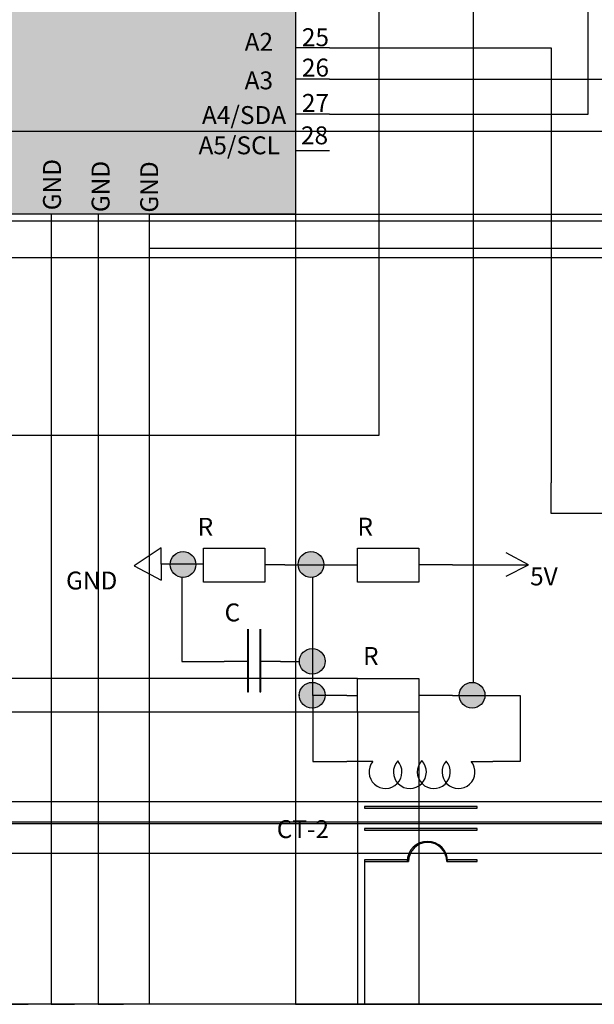
# Model space of a CAD drawing. Units: inches. Extents: x 35362 to 73946, y 43607 to 67532.
# Tile 133 of 134: x 57838 to 64925, y 43607 to 55752. Entities that reach past the tile are written whole.
import ezdxf

# ---------------------------------------------------------------- set-up
doc = ezdxf.new("R2010")
doc.units = ezdxf.units.IN
doc.header["$MEASUREMENT"] = 0
for name, color, linetype, lineweight in [('A-ANNO-DIMS', 2, 'Continuous', 18), ('E-ANNO-TEXT', 5, 'Continuous', 18), ('E-SYMB', 1, 'Continuous', 25), ('E-SYMB-PATT', 1, 'Continuous', 13), ('E-WIRE', 3, 'Continuous', 25)]:
    doc.layers.add(name, color=color, linetype=linetype, lineweight=lineweight)
doc.styles.get("Standard").update_dxf_attribs({"font": 'arial.ttf'})
doc.dimstyles.get("Standard").update_dxf_attribs({"dimtxt": 0.18, "dimasz": 0.18, "dimexe": 0.18, "dimexo": 0.0625, "dimgap": 0.09, "dimtad": 0, "dimtih": 1, "dimtoh": 1, "dimdec": 4, "dimzin": 0, "dimdsep": 46, "dimtxsty": 'Standard', "dimcen": 0.09, "dimadec": 0, "dimazin": 0, "dimtfac": 1, "dimtdec": 4, "dimtofl": 0, "dimtmove": 0, "dimatfit": 3, "dimfxl": 1, "dimtolj": 1, "dimtzin": 0, "dimarcsym": 0})

# ---------------------------------------------------------------- blocks, each defined once
blk = doc.blocks.new('CT-CORE')
for p, q in [((-0.0004610742907971, 1387.996120092102), (-0.0004610742907971, -5.34733626409e-05)), ((19.99953892572375, 1387.996120092102), (-0.0004610742907971, 1387.996120092102)), ((19.9995389257092, -5.34733626409e-05), (19.99953892572375, 1387.996120092102)), ((270.6681283192447, 1387.996120092102), (270.6681283192447, -5.34733626409e-05)), ((290.6681283192593, 1387.996120092102), (270.6681283192447, 1387.996120092102)), ((290.6681283192447, -5.34733626409e-05), (290.6681283192593, 1387.996120092102)), ((658.9826659540267, 1387.996120092102), (658.9826659540267, 1014.585417332389)), ((678.9826659540413, 1387.996120092102), (658.9826659540267, 1387.996120092102)), ((678.9826659540413, 1015.434583844784), (678.9826659540413, 1387.996120092102)), ((658.9826659540267, 544.3844491987692), (658.9826659540267, -5.34733626409e-05)), ((678.9826659540267, -5.34733626409e-05), (678.9826659540413, 543.5352826863744)), ((-0.0004610742907971, -5.34733626409e-05), (19.9995389257092, -5.34733626409e-05)), ((270.6681283192447, -5.34733626409e-05), (290.6681283192447, -5.34733626409e-05)), ((658.9826659540267, -5.34733626409e-05), (678.9826659540267, -5.34733626409e-05))]:
    blk.add_line(p, q)
blk.add_arc((678.9826659540267, 779.4849332655793), 235.9496505792049, 90, 270)
blk = doc.blocks.new('PWR-5V')
for p, q in [((149.83075954589, 1350.920325582869), (-0.0001436721213395, 1075.898385659784)), ((149.83075954589, 833.0941938853575), (149.83075954589, 1350.920325582869)), ((289.9554714129044, 1075.898385659784), (149.83075954589, 1350.920325582869)), ((149.83075954589, 416.3126341884199), (149.83075954589, 833.0941938853575)), ((149.83075954589, 416.3126341884199), (149.83075954589, 0.0003315384019515))]:
    blk.add_line(p, q)
blk = doc.blocks.new('*D5')
at = {"layer": 'A-ANNO-DIMS', "color": 0, "lineweight": -2, "transparency": 16777216}
for p, q in [((37121.949085, 46919.318283), (37121.949085, 43606.678996)), ((69871.496302, 45449.831951), (69871.496302, 43606.678996)), ((37122.129085, 43606.858996), (53496.2943647142, 43606.858996)), ((69871.316302, 43606.858996), (53497.15102228581, 43606.858996))]:
    blk.add_line(p, q, dxfattribs=at)
at = {"layer": 'A-ANNO-DIMS', "color": 0, "transparency": 16777216}
for points in [[(37122.129085, 43606.888996), (37122.129085, 43606.828996), (37121.949085, 43606.858996)], [(69871.316302, 43606.888996), (69871.316302, 43606.828996), (69871.496302, 43606.858996)]]:
    blk.add_solid(points, dxfattribs=at)
at = {"layer": 'Defpoints', "color": 0, "transparency": 16777216}
for p in [(37121.949085, 46919.380783), (69871.496302, 45449.894451), (69871.496302, 43606.858996)]:
    blk.add_point(p, dxfattribs=at)
at = {"layer": 'A-ANNO-DIMS', "color": 0, "transparency": 16777216, "insert": (53496.7226935, 43606.858996), "char_height": 0.18, "attachment_point": 5}
blk.add_mtext('\\A1;32750', dxfattribs=at)
blk = doc.blocks.new('*D10')
at = {"layer": 'A-ANNO-DIMS', "color": 0, "lineweight": -2, "transparency": 16777216}
for p, q in [((61240.96983600002, 59185.14395700003), (73945.82566600003, 59185.14395700003)), ((73945.64566600005, 59184.96395700003), (73945.64566600005, 56268.51827402935)), ((73945.64566600005, 53351.70866200003), (73945.64566600005, 56268.1543449707)), ((61240.96983600002, 53351.52866200003), (73945.82566600003, 53351.52866200003))]:
    blk.add_line(p, q, dxfattribs=at)
at = {"layer": 'A-ANNO-DIMS', "color": 0, "transparency": 16777216}
for points in [[(73945.61566600006, 59184.96395700003), (73945.67566600005, 59184.96395700003), (73945.64566600005, 59185.14395700003)], [(73945.61566600006, 53351.70866200003), (73945.67566600005, 53351.70866200003), (73945.64566600005, 53351.52866200003)]]:
    blk.add_solid(points, dxfattribs=at)
at = {"layer": 'Defpoints', "color": 0, "transparency": 16777216}
for p in [(61240.90733600002, 59185.14395700003), (61240.90733600002, 53351.52866200003), (73945.64566600005, 53351.52866200003)]:
    blk.add_point(p, dxfattribs=at)
at = {"layer": 'A-ANNO-DIMS', "color": 0, "transparency": 16777216, "insert": (73945.64566600005, 56268.33630949999), "char_height": 0.18, "attachment_point": 5}
blk.add_mtext('\\A1;5834', dxfattribs=at)
blk = doc.blocks.new('*D36')
at = {"layer": 'A-ANNO-DIMS', "color": 0, "lineweight": -2, "transparency": 16777216}
for p, q in [((68320.80826200004, 60122.34633200002), (35361.76908500003, 60122.34633200002)), ((35361.94908500003, 60122.16633200002), (35361.94908500003, 57247.82893113781)), ((35361.94908500003, 54373.12772400002), (35361.94908500003, 57247.46512486223)), ((68320.80826200004, 54372.94772400003), (35361.76908500003, 54372.94772400002))]:
    blk.add_line(p, q, dxfattribs=at)
at = {"layer": 'A-ANNO-DIMS', "color": 0, "transparency": 16777216}
for points in [[(35361.91908500003, 60122.16633200002), (35361.97908500003, 60122.16633200002), (35361.94908500003, 60122.34633200002)], [(35361.91908500003, 54373.12772400002), (35361.97908500003, 54373.12772400002), (35361.94908500003, 54372.94772400002)]]:
    blk.add_solid(points, dxfattribs=at)
at = {"layer": 'Defpoints', "color": 0, "transparency": 16777216}
for p in [(68320.87076200004, 60122.34633200002), (35361.94908500003, 54372.94772400002), (68320.87076200004, 54372.94772400003)]:
    blk.add_point(p, dxfattribs=at)
at = {"layer": 'A-ANNO-DIMS', "color": 0, "transparency": 16777216, "insert": (35361.94908500004, 57247.64702799999), "char_height": 0.18, "attachment_point": 5}
blk.add_mtext('\\A1;5749.4', dxfattribs=at)
blk = doc.blocks.new('*D37')
at = {"layer": 'A-ANNO-DIMS', "color": 0, "lineweight": -2, "transparency": 16777216}
for p, q in [((53793.637789, 45449.831951), (53793.637789, 43606.678996)), ((62090.58505699999, 45366.796496), (62090.58505699999, 43606.678996)), ((53793.817789, 43606.858996), (57941.64748712004, 43606.858996)), ((62090.40505699999, 43606.858996), (57942.57535887994, 43606.858996))]:
    blk.add_line(p, q, dxfattribs=at)
at = {"layer": 'A-ANNO-DIMS', "color": 0, "transparency": 16777216}
for points in [[(53793.817789, 43606.888996), (53793.817789, 43606.828996), (53793.637789, 43606.858996)], [(62090.40505699999, 43606.888996), (62090.40505699999, 43606.828996), (62090.58505699999, 43606.858996)]]:
    blk.add_solid(points, dxfattribs=at)
at = {"layer": 'Defpoints', "color": 0, "transparency": 16777216}
for p in [(53793.637789, 45449.894451), (62090.58505699999, 45366.858996), (62090.58505699999, 43606.858996)]:
    blk.add_point(p, dxfattribs=at)
at = {"layer": 'A-ANNO-DIMS', "color": 0, "transparency": 16777216, "insert": (57942.111423, 43606.858996), "char_height": 0.18, "attachment_point": 5}
blk.add_mtext('\\A1;8296.9', dxfattribs=at)
blk = doc.blocks.new('*D38')
at = {"layer": 'A-ANNO-DIMS', "color": 0, "lineweight": -2, "transparency": 16777216}
for p, q in [((68483.500128, 45449.831951), (68483.500128, 43606.678996)), ((62090.58505699999, 45366.796496), (62090.58505699999, 43606.678996)), ((62090.76505699999, 43606.858996), (65286.57828827081, 43606.858996)), ((68483.320128, 43606.858996), (65287.5068967292, 43606.858996))]:
    blk.add_line(p, q, dxfattribs=at)
at = {"layer": 'A-ANNO-DIMS', "color": 0, "transparency": 16777216}
for points in [[(62090.76505699999, 43606.888996), (62090.76505699999, 43606.828996), (62090.58505699999, 43606.858996)], [(68483.320128, 43606.888996), (68483.320128, 43606.828996), (68483.500128, 43606.858996)]]:
    blk.add_solid(points, dxfattribs=at)
at = {"layer": 'Defpoints', "color": 0, "transparency": 16777216}
for p in [(68483.500128, 45449.894451), (62090.58505699999, 45366.858996), (68483.500128, 43606.858996)]:
    blk.add_point(p, dxfattribs=at)
at = {"layer": 'A-ANNO-DIMS', "color": 0, "transparency": 16777216, "insert": (65287.0425925, 43606.858996), "char_height": 0.18, "attachment_point": 5}
blk.add_mtext('\\A1;6392.9', dxfattribs=at)
blk = doc.blocks.new('*D42')
at = {"layer": 'A-ANNO-DIMS', "color": 0, "lineweight": -2, "transparency": 16777216}
for p, q in [((62004.728148, 47208.187381), (62004.728148, 43606.678996)), ((62761.346442, 47208.187381), (62761.346442, 43606.678996)), ((62004.908148, 43606.858996), (62382.64438913369, 43606.858996)), ((62761.166442, 43606.858996), (62383.43020086631, 43606.858996))]:
    blk.add_line(p, q, dxfattribs=at)
at = {"layer": 'A-ANNO-DIMS', "color": 0, "transparency": 16777216}
for points in [[(62004.908148, 43606.888996), (62004.908148, 43606.828996), (62004.728148, 43606.858996)], [(62761.166442, 43606.888996), (62761.166442, 43606.828996), (62761.346442, 43606.858996)]]:
    blk.add_solid(points, dxfattribs=at)
at = {"layer": 'Defpoints', "color": 0, "transparency": 16777216}
for p in [(62004.728148, 47208.249881), (62761.346442, 47208.249881), (62761.346442, 43606.858996)]:
    blk.add_point(p, dxfattribs=at)
at = {"layer": 'A-ANNO-DIMS', "color": 0, "transparency": 16777216, "insert": (62383.037295, 43606.858996), "char_height": 0.18, "attachment_point": 5}
blk.add_mtext('\\A1;756.6', dxfattribs=at)
blk = doc.blocks.new('*D43')
at = {"layer": 'A-ANNO-DIMS', "color": 0, "lineweight": -2, "transparency": 16777216}
for p, q in [((62004.66564800003, 47625.18100000001), (35361.76908500003, 47625.181)), ((35361.94908500003, 47625.001), (35361.94908500003, 47416.89734363779)), ((35361.94908500003, 47208.42988100001), (35361.94908500003, 47416.53353736221)), ((62004.66564800003, 47208.24988100002), (35361.76908500003, 47208.24988100001))]:
    blk.add_line(p, q, dxfattribs=at)
at = {"layer": 'A-ANNO-DIMS', "color": 0, "transparency": 16777216}
for points in [[(35361.91908500003, 47625.001), (35361.97908500003, 47625.001), (35361.94908500003, 47625.181)], [(35361.91908500003, 47208.42988100001), (35361.97908500003, 47208.42988100001), (35361.94908500003, 47208.24988100001)]]:
    blk.add_solid(points, dxfattribs=at)
at = {"layer": 'Defpoints', "color": 0, "transparency": 16777216}
for p in [(62004.72814800003, 47625.18100000001), (35361.94908500003, 47208.24988100001), (62004.72814800003, 47208.24988100002)]:
    blk.add_point(p, dxfattribs=at)
at = {"layer": 'A-ANNO-DIMS', "color": 0, "transparency": 16777216, "insert": (35361.94908500003, 47416.71544049999), "char_height": 0.18, "attachment_point": 5}
blk.add_mtext('\\A1;416.9', dxfattribs=at)
blk = doc.blocks.new('*D53')
at = {"layer": 'A-ANNO-DIMS', "color": 0, "lineweight": -2, "transparency": 16777216}
for p, q in [((56873.601939, 53351.466162), (56873.601939, 43606.678996)), ((58224.785482, 52935.15386), (58224.785482, 43606.678996)), ((56873.78193899999, 43606.858996), (57548.73947448363, 43606.858996)), ((58224.605482, 43606.858996), (57549.64794651637, 43606.858996))]:
    blk.add_line(p, q, dxfattribs=at)
at = {"layer": 'A-ANNO-DIMS', "color": 0, "transparency": 16777216}
for points in [[(56873.78193899999, 43606.888996), (56873.78193899999, 43606.828996), (56873.601939, 43606.858996)], [(58224.605482, 43606.888996), (58224.605482, 43606.828996), (58224.785482, 43606.858996)]]:
    blk.add_solid(points, dxfattribs=at)
at = {"layer": 'Defpoints', "color": 0, "transparency": 16777216}
for p in [(56873.601939, 53351.52866199999), (58224.785482, 52935.21636), (58224.785482, 43606.858996)]:
    blk.add_point(p, dxfattribs=at)
at = {"layer": 'A-ANNO-DIMS', "color": 0, "transparency": 16777216, "insert": (57549.19371049999, 43606.858996), "char_height": 0.18, "attachment_point": 5}
blk.add_mtext('\\A1;1351.2', dxfattribs=at)
blk = doc.blocks.new('*D54')
at = {"layer": 'A-ANNO-DIMS', "color": 0, "lineweight": -2, "transparency": 16777216}
for p, q in [((58224.785482, 52935.15386), (58224.785482, 43606.678996)), ((58805.728279, 52935.15386), (58805.728279, 43606.678996)), ((58224.965482, 43606.858996), (58514.86299236904, 43606.858996)), ((58805.548279, 43606.858996), (58515.65076863097, 43606.858996))]:
    blk.add_line(p, q, dxfattribs=at)
at = {"layer": 'A-ANNO-DIMS', "color": 0, "transparency": 16777216}
for points in [[(58224.965482, 43606.888996), (58224.965482, 43606.828996), (58224.785482, 43606.858996)], [(58805.548279, 43606.888996), (58805.548279, 43606.828996), (58805.728279, 43606.858996)]]:
    blk.add_solid(points, dxfattribs=at)
at = {"layer": 'Defpoints', "color": 0, "transparency": 16777216}
for p in [(58224.785482, 52935.21636), (58805.728279, 52935.21636), (58805.728279, 43606.858996)]:
    blk.add_point(p, dxfattribs=at)
at = {"layer": 'A-ANNO-DIMS', "color": 0, "transparency": 16777216, "insert": (58515.2568805, 43606.858996), "char_height": 0.18, "attachment_point": 5}
blk.add_mtext('\\A1;580.9', dxfattribs=at)
blk = doc.blocks.new('*D55')
at = {"layer": 'A-ANNO-DIMS', "color": 0, "lineweight": -2, "transparency": 16777216}
for p, q in [((58805.728279, 52935.15386), (58805.728279, 43606.678996)), ((59433.145179, 52935.15386), (59433.145179, 43606.678996)), ((58805.908279, 43606.858996), (59119.04290226058, 43606.858996)), ((59432.965179, 43606.858996), (59119.83055573942, 43606.858996))]:
    blk.add_line(p, q, dxfattribs=at)
at = {"layer": 'A-ANNO-DIMS', "color": 0, "transparency": 16777216}
for points in [[(58805.908279, 43606.888996), (58805.908279, 43606.828996), (58805.728279, 43606.858996)], [(59432.965179, 43606.888996), (59432.965179, 43606.828996), (59433.145179, 43606.858996)]]:
    blk.add_solid(points, dxfattribs=at)
at = {"layer": 'Defpoints', "color": 0, "transparency": 16777216}
for p in [(58805.728279, 52935.21636), (59433.145179, 52935.21636), (59433.145179, 43606.858996)]:
    blk.add_point(p, dxfattribs=at)
at = {"layer": 'A-ANNO-DIMS', "color": 0, "transparency": 16777216, "insert": (59119.436729, 43606.858996), "char_height": 0.18, "attachment_point": 5}
blk.add_mtext('\\A1;627.4', dxfattribs=at)
blk = doc.blocks.new('*D56')
at = {"layer": 'A-ANNO-DIMS', "color": 0, "lineweight": -2, "transparency": 16777216}
for p, q in [((59433.20767900003, 53351.52866200003), (73945.82566600003, 53351.52866200003)), ((73945.64566600005, 53351.34866200002), (73945.64566600005, 53143.55447552935)), ((73945.64566600005, 52935.39636000002), (73945.64566600005, 53143.19054647069)), ((59433.20767900003, 52935.21636000003), (73945.82566600003, 52935.21636000003))]:
    blk.add_line(p, q, dxfattribs=at)
at = {"layer": 'A-ANNO-DIMS', "color": 0, "transparency": 16777216}
for points in [[(73945.61566600006, 53351.34866200002), (73945.67566600005, 53351.34866200002), (73945.64566600005, 53351.52866200003)], [(73945.61566600006, 52935.39636000002), (73945.67566600005, 52935.39636000002), (73945.64566600005, 52935.21636000003)]]:
    blk.add_solid(points, dxfattribs=at)
at = {"layer": 'Defpoints', "color": 0, "transparency": 16777216}
for p in [(59433.14517900002, 53351.52866200003), (59433.14517900002, 52935.21636000003), (73945.64566600005, 52935.21636000003)]:
    blk.add_point(p, dxfattribs=at)
at = {"layer": 'A-ANNO-DIMS', "color": 0, "transparency": 16777216, "insert": (73945.64566600005, 53143.37251099998), "char_height": 0.18, "attachment_point": 5}
blk.add_mtext('\\A1;416.3', dxfattribs=at)
blk = doc.blocks.new('*D57')
at = {"layer": 'A-ANNO-DIMS', "color": 0, "lineweight": -2, "transparency": 16777216}
for p, q in [((51445.41811300003, 53272.78194700003), (73945.82566600003, 53272.78194700003)), ((73945.64566600005, 53272.60194700003), (73945.64566600005, 53045.85764863782)), ((73945.64566600005, 52818.74954400002), (73945.64566600005, 53045.49384236224)), ((51445.41811300003, 52818.56954400002), (73945.82566600003, 52818.56954400002))]:
    blk.add_line(p, q, dxfattribs=at)
at = {"layer": 'A-ANNO-DIMS', "color": 0, "transparency": 16777216}
for points in [[(73945.61566600006, 53272.60194700003), (73945.67566600005, 53272.60194700003), (73945.64566600005, 53272.78194700003)], [(73945.61566600006, 52818.74954400002), (73945.67566600005, 52818.74954400002), (73945.64566600005, 52818.56954400002)]]:
    blk.add_solid(points, dxfattribs=at)
at = {"layer": 'Defpoints', "color": 0, "transparency": 16777216}
for p in [(51445.35561300003, 53272.78194700003), (51445.35561300003, 52818.56954400002), (73945.64566600005, 52818.56954400002)]:
    blk.add_point(p, dxfattribs=at)
at = {"layer": 'A-ANNO-DIMS', "color": 0, "transparency": 16777216, "insert": (73945.64566600005, 53045.6757455), "char_height": 0.18, "attachment_point": 5}
blk.add_mtext('\\A1;454.2', dxfattribs=at)
blk = doc.blocks.new('*D68')
at = {"layer": 'A-ANNO-DIMS', "color": 0, "lineweight": -2, "transparency": 16777216}
for p, q in [((68320.870762, 54372.885224), (68320.870762, 43606.678996)), ((61240.907336, 53351.466162), (61240.907336, 43606.678996)), ((61241.08733599999, 43606.858996), (64780.42646373397, 43606.858996)), ((68320.69076200001, 43606.858996), (64781.35163426603, 43606.858996))]:
    blk.add_line(p, q, dxfattribs=at)
at = {"layer": 'A-ANNO-DIMS', "color": 0, "transparency": 16777216}
for points in [[(61241.08733599999, 43606.888996), (61241.08733599999, 43606.828996), (61240.907336, 43606.858996)], [(68320.69076200001, 43606.888996), (68320.69076200001, 43606.828996), (68320.870762, 43606.858996)]]:
    blk.add_solid(points, dxfattribs=at)
at = {"layer": 'Defpoints', "color": 0, "transparency": 16777216}
for p in [(68320.870762, 54372.947724), (61240.907336, 53351.52866199999), (68320.870762, 43606.858996)]:
    blk.add_point(p, dxfattribs=at)
at = {"layer": 'A-ANNO-DIMS', "color": 0, "transparency": 16777216, "insert": (64780.889049, 43606.858996), "char_height": 0.18, "attachment_point": 5}
blk.add_mtext('\\A1;7080.0', dxfattribs=at)
blk = doc.blocks.new('*D74')
at = {"layer": 'A-ANNO-DIMS', "color": 0, "lineweight": -2, "transparency": 16777216}
for p, q in [((55181.69646300003, 46108.87757800001), (73945.82566600003, 46108.87757800001)), ((73945.64566600005, 46108.69757800001), (73945.64566600005, 45983.7251866378)), ((73945.64566600005, 45858.38898900001), (73945.64566600005, 45983.36138036223)), ((55181.69646300003, 45858.20898900001), (73945.82566600003, 45858.20898900001))]:
    blk.add_line(p, q, dxfattribs=at)
at = {"layer": 'A-ANNO-DIMS', "color": 0, "transparency": 16777216}
for points in [[(73945.61566600006, 46108.69757800001), (73945.67566600005, 46108.69757800001), (73945.64566600005, 46108.87757800001)], [(73945.61566600006, 45858.38898900001), (73945.67566600005, 45858.38898900001), (73945.64566600005, 45858.20898900001)]]:
    blk.add_solid(points, dxfattribs=at)
at = {"layer": 'Defpoints', "color": 0, "transparency": 16777216}
for p in [(55181.63396300002, 46108.87757800001), (55181.63396300002, 45858.20898900001), (73945.64566600005, 45858.20898900001)]:
    blk.add_point(p, dxfattribs=at)
at = {"layer": 'A-ANNO-DIMS', "color": 0, "transparency": 16777216, "insert": (73945.64566600005, 45983.54328349999), "char_height": 0.18, "attachment_point": 5}
blk.add_mtext('\\A1;250.67', dxfattribs=at)
blk = doc.blocks.new('*D75')
at = {"layer": 'A-ANNO-DIMS', "color": 0, "lineweight": -2, "transparency": 16777216}
for p, q in [((55181.69646300003, 45838.20898900001), (73945.82566600003, 45838.20898900001)), ((73945.64566600005, 45838.02898900001), (73945.64566600005, 45654.23368452933)), ((73945.64566600005, 45470.07445100001), (73945.64566600005, 45653.86975547068)), ((55181.69646300003, 45469.89445100001), (73945.82566600003, 45469.89445100001))]:
    blk.add_line(p, q, dxfattribs=at)
at = {"layer": 'A-ANNO-DIMS', "color": 0, "transparency": 16777216}
for points in [[(73945.61566600006, 45838.02898900001), (73945.67566600005, 45838.02898900001), (73945.64566600005, 45838.20898900001)], [(73945.61566600006, 45470.07445100001), (73945.67566600005, 45470.07445100001), (73945.64566600005, 45469.89445100001)]]:
    blk.add_solid(points, dxfattribs=at)
at = {"layer": 'Defpoints', "color": 0, "transparency": 16777216}
for p in [(55181.63396300002, 45838.20898900001), (55181.63396300002, 45469.89445100001), (73945.64566600005, 45469.89445100001)]:
    blk.add_point(p, dxfattribs=at)
at = {"layer": 'A-ANNO-DIMS', "color": 0, "transparency": 16777216, "insert": (73945.64566600005, 45654.05171999998), "char_height": 0.18, "attachment_point": 5}
blk.add_mtext('\\A1;368.3', dxfattribs=at)

msp = doc.modelspace()

# ---------------------------------------------------------------- hatches: boundary and pattern name
at = {"layer": 'E-SYMB-PATT'}
h = msp.add_hatch(color=256, dxfattribs=at)
h.dxf.hatch_style = 1
h.paths.add_polyline_path([(56873.60193850077, 59185.14395657572), (56873.60193850077, 53351.5286622623), (61240.90733594325, 53351.5286622623), (61240.90733594325, 59185.14395657572)])
h = msp.add_hatch(color=256, dxfattribs=at)
h.dxf.hatch_style = 1
h.paths.add_polyline_path([(60011.21456379792, 49029.51137446792, 0.4183931940818975), (59852.62477841939, 49190.37716580508, 0.4183931940818975), (59694.03499304087, 49029.51137446792)])
h.paths.add_polyline_path([(60011.21456379792, 49029.51137446792), (59694.03499304087, 49029.51137446792, 0.4100462469397049), (59852.62477841939, 48873.16539302992, 0.4100462469397049)])
h = msp.add_hatch(color=256, dxfattribs=at)
h.dxf.hatch_style = 1
h.paths.add_polyline_path([(61589.1028690778, 49029.51137446792, 0.4183931940818975), (61430.51308369927, 49190.37716580508, 0.4183931940818975), (61271.92329832073, 49029.51137446792)])
h.paths.add_polyline_path([(61589.1028690778, 49029.51137446792), (61271.92329832073, 49029.51137446792, 0.4100462469397049), (61430.51308369927, 48873.16539302992, 0.4100462469397049)])
h = msp.add_hatch(color=256, dxfattribs=at)
h.dxf.hatch_style = 1
h.paths.add_polyline_path([(60648.34921623781, 47461.09843796286), (60659.50392597078, 47461.09843796286), (60659.50392597078, 48235.23315929426), (60648.34921623781, 48235.23315929426)])
h = msp.add_hatch(color=256, dxfattribs=at)
h.dxf.hatch_style = 1
h.paths.add_polyline_path([(60799.31069366398, 47461.09843796286), (60810.46540339697, 47461.09843796286), (60810.46540339697, 48235.23315929426), (60799.31069366398, 48235.23315929426)])
h = msp.add_hatch(color=256, dxfattribs=at)
h.dxf.hatch_style = 1
h.paths.add_polyline_path([(61604.31868538361, 47835.05338572362, 0.4183931940818975), (61445.72890000508, 47995.91917706077, 0.4183931940818975), (61287.13911462654, 47835.05338572362)])
h.paths.add_polyline_path([(61604.31868538361, 47835.05338572362), (61287.13911462654, 47835.05338572362, 0.4100462469397049), (61445.72890000508, 47678.70740428561, 0.4100462469397049)])
h = msp.add_hatch(color=256, dxfattribs=at)
h.dxf.hatch_style = 1
h.paths.add_polyline_path([(61604.03314156829, 47416.69937334141, 0.4183931940818975), (61445.44335618975, 47577.56516467857, 0.4183931940818975), (61286.85357081121, 47416.69937334141)])
h.paths.add_polyline_path([(61604.03314156829, 47416.69937334141), (61286.85357081121, 47416.69937334141, 0.4100462469397049), (61445.44335618975, 47260.35339190341, 0.4100462469397049)])
h = msp.add_hatch(color=256, dxfattribs=at)
h.dxf.hatch_style = 1
h.paths.add_polyline_path([(63576.48012757601, 47416.69937334139, 0.4183931940818975), (63417.89034219747, 47577.56516467855, 0.4183931940818975), (63259.30055681894, 47416.69937334139)])
h.paths.add_polyline_path([(63576.48012757601, 47416.69937334139), (63259.30055681894, 47416.69937334139, 0.4100462469397049), (63417.89034219747, 47260.35339190339, 0.4100462469397049)])
h = msp.add_hatch(color=256, dxfattribs=at)
h.dxf.hatch_style = 1
h.paths.add_polyline_path([(63478.5812302799, 46025.84212335861), (63478.5812302799, 46045.84212335862), (62090.58505671445, 46045.84212335862), (62090.58505671445, 46025.84212335862)])
h = msp.add_hatch(color=256, dxfattribs=at)
h.dxf.hatch_style = 1
h.paths.add_polyline_path([(63478.5812302799, 45755.17353396508), (63478.5812302799, 45775.17353396509), (62090.58505671445, 45775.17353396509), (62090.58505671445, 45755.17353396509)])
h = msp.add_hatch(color=256, dxfattribs=at)
h.dxf.hatch_style = 1
h.paths.add_polyline_path([(63105.17052752019, 45386.85899633031), (63115.32647614845, 45386.85899633031, 0.3908929169039177), (62866.71156053301, 45616.27707159044, 0.3908929169039177), (62618.09664491756, 45386.85899633031), (62634.96955938657, 45386.85899633031, -0.389569854577291), (62870.0700434534, 45602.80864690951, -0.389569854577291)])
h = msp.add_hatch(color=256, dxfattribs=at)
h.dxf.hatch_style = 1
h.paths.add_polyline_path([(62634.12039287417, 45366.85899633029, -0.0212196039209565), (62634.96955938657, 45386.85899633031), (62618.09664491756, 45386.85899633031, 0.0200709024740955), (62617.29348527288, 45366.85899633029)])
h.paths.add_polyline_path([(62617.29348527288, 45366.85899633029, -0.0200709024740953), (62618.09664491756, 45386.85899633031), (62090.58505671445, 45386.85899633031), (62090.58505671445, 45366.85899633031)])
h.paths.add_polyline_path([(63478.5812302799, 45366.85899633029), (63478.5812302799, 45386.85899633031), (63115.32647614845, 45386.85899633031, -0.0200709024740959), (63116.12963579316, 45366.85899633029)])
h.paths.add_polyline_path([(63116.12963579316, 45366.85899633029, 0.020070902474096), (63115.32647614845, 45386.85899633031), (63105.17052752019, 45386.85899633031, -0.0212196039209564), (63106.01969403259, 45366.85899633029)])

# ---------------------------------------------------------------- linework, layer by layer
at = {"layer": 'E-SYMB'}
for p, q in [((61657.21963859326, 55403.03834364471), (61240.90733594325, 55403.03834364471)), ((61657.21963859326, 55020.33824525718), (61240.90733594325, 55020.33824525718)), ((61657.21963859326, 54587.23758632809), (61240.90733594325, 54587.23758632809)), ((61657.21963859326, 54135.79828039984), (61240.90733594325, 54135.79828039984)), ((58224.78548248348, 53351.5286622623), (58224.78548248348, 52935.21635961227)), ((58805.72827947429, 53351.5286622623), (58805.72827947429, 52935.21635961227)), ((59433.1451794252, 53351.5286622623), (59433.1451794252, 52935.21635961227)), ((59582.54222905269, 49237.04367651214), (59249.60924639129, 49015.33298877657)), ((59582.54222905269, 49037.04367651214), (59582.54222905269, 49237.04367651214)), ((59249.60924639129, 49015.33298877657), (59582.54222905269, 48837.04367651214)), ((60011.14300773598, 49037.04367651214), (59582.54222905269, 49037.04367651214)), ((59582.54222905269, 49037.04367651214), (59582.54222905269, 48837.04367651214)), ((59698.50613852575, 49029.51137446792), (59694.03499304087, 49029.51137446792)), ((60011.2137633826, 49034.08667250018), (60010.52754012158, 49034.08667250018)), ((60103.46384748086, 49037.04367651214), (60011.14300773598, 49037.04367651214)), ((61107.38135627366, 49029.51137446792), (60860.08214115561, 49029.51137446792)), ((61276.39444380563, 49029.51137446792), (61271.92329832073, 49029.51137446792)), ((61589.10206866248, 49034.08667250018), (61588.41584540144, 49034.08667250018)), ((61734.61245421725, 49029.51137446792), (62004.72814805145, 49029.51137446792)), ((60648.34921623781, 48235.23315929426), (60648.34921623781, 47461.09843796286)), ((60659.50392597078, 47461.09843796286), (60659.50392597078, 48235.23315929426)), ((60799.31069366398, 48235.23315929426), (60799.31069366398, 47461.09843796286)), ((60810.46540339697, 47461.09843796286), (60810.46540339697, 48235.23315929426)), ((60659.50392597078, 47835.0533857236), (60357.94878666321, 47835.05338572362)), ((61053.54433516212, 47835.05338572362), (60799.31069366398, 47835.0533857236)), ((61291.61026011144, 47835.05338572362), (61287.13911462654, 47835.05338572362)), ((61604.31788496828, 47839.62868375587), (61603.63166170724, 47839.62868375587)), ((60648.34921623781, 47461.09843796286), (60659.50392597078, 47461.09843796286)), ((60799.31069366398, 47461.09843796286), (60810.46540339697, 47461.09843796286)), ((61291.32471629612, 47416.69937334141), (61286.85357081121, 47416.69937334141)), ((61604.03234115297, 47421.27467137366), (61603.34611789192, 47421.27467137366)), ((61871.80981872411, 47416.69937334141), (62004.72814805145, 47416.10587040346)), ((63177.65874437623, 47416.69937334139), (62761.3464417262, 47416.69937334139)), ((63263.77170230384, 47416.69937334139), (63259.30055681894, 47416.69937334139)), ((63576.47932716069, 47421.27467137366), (63575.79310389964, 47421.27467137366)), ((61994.50760290873, 46600.5876377495), (61871.80981872411, 46600.5876377495)), ((62192.12464685281, 46600.5876377495), (61994.50760290873, 46600.5876377495)), ((62507.56875075863, 46600.5876377495), (62492.30534187303, 46600.5876377495)), ((62807.74944577881, 46600.5876377495), (62787.3981698774, 46600.5876377495)), ((63102.84227378319, 46600.5876377495), (63092.66663583252, 46600.5876377495)), ((63408.11073973831, 46600.5876377495), (63674.31243090352, 46600.5876377495))]:
    msp.add_line(p, q, dxfattribs=at)
for points in [[(56873.60193850077, 59185.14395657572), (61240.90733594325, 59185.14395657572), (61240.90733594325, 53351.5286622623), (56873.60193850077, 53351.5286622623)], [(60860.08214115561, 49231.63390007417), (60860.08214115561, 48814.70278119428), (60103.46384748086, 48814.70278119428), (60103.46384748086, 49231.63390007417)], [(62761.3464417262, 49231.63390007417), (62761.3464417262, 48814.70278119428), (62004.72814805145, 48814.70278119428), (62004.72814805145, 49231.63390007417)], [(62761.3464417262, 47625.18099956924), (62761.3464417262, 47208.24988068935), (62004.72814805145, 47208.24988068935), (62004.72814805145, 47625.18099956924)]]:
    msp.add_lwpolyline(points, close=True, dxfattribs=at)
for centre in [(59852.62477841939, 49031.7712794175), (61430.51308369927, 49031.7712794175), (61445.72890000508, 47837.31329067319), (61445.44335618975, 47418.95927829099), (63417.89034219747, 47418.95927829097)]:
    msp.add_circle(centre, 158.6058863875805, dxfattribs=at)
for centre, radius, start, end in [((62349.84669880572, 46472.25797890667), 203.3340773479672, 140.866668573025, 42.42623157979358), ((62650.02739382592, 46472.25797890667), 203.3340773479672, 137.5737684202064, 43.47826481578265), ((62945.12022183029, 46472.25797890667), 203.3340773479672, 136.5217351842173, 41.35264262444016), ((63250.3886877854, 46472.25797890667), 203.3340773479672, 138.6473573755598, 39.13333142697496), ((62866.71156053301, 45366.85899633031), 249.4180752601387, 0, 180)]:
    msp.add_arc(centre, radius, start, end, dxfattribs=at)
at = {"layer": 'E-WIRE'}
for p, q in [((64849.63466818351, 54587.23758632809), (64849.6346681835, 59750.68874003685)), ((62267.52571652509, 56394.41825037897), (62267.52571652509, 50624.74016954905)), ((63433.66154480785, 47576.77910076272), (63433.66154480784, 55899.60469189059)), ((61657.21963859326, 55403.03834364471), (64391.6881470991, 55403.03834364471)), ((64391.6881470991, 55403.03834364471), (64391.6881470991, 50581.64775167532)), ((61657.21963859326, 55020.33824525718), (70677.18977032776, 55020.33824525718)), ((61657.21963859326, 54587.23758632809), (64849.63466818351, 54587.23758632809)), ((62267.52571652509, 50624.74016954905), (55134.81271077293, 50624.74016954904)), ((64391.6881470991, 50581.64775167532), (64391.6881470991, 50038.84084173529)), ((64391.6881470991, 49659.17196353645), (64391.6881470991, 50038.84084173529)), ((69802.97030670266, 49659.17196353646), (64391.6881470991, 49659.17196353645)), ((61107.38135627366, 49029.51137446792), (61734.61245421725, 49029.51137446792)), ((59837.49838463528, 48873.88834997965), (59837.49838463528, 47835.05338572364)), ((61451.79487336342, 47416.69937334141), (61452.79004443131, 48874.73763901732)), ((59837.49838463528, 47835.05338572364), (60357.94878666321, 47835.05338572362)), ((61053.54433516212, 47835.05338572362), (61287.13911462654, 47835.05338572362)), ((61871.80981872411, 47416.69937334141), (61451.79487336342, 47416.69937334141)), ((61451.79487336342, 47416.69937334141), (61451.79487336342, 46600.5876377495)), ((63177.65874437623, 47416.69937334139), (63594.44030407315, 47416.69937334139)), ((63594.44030407315, 47416.69937334139), (64009.18616959618, 47416.69937334139)), ((64009.18616959618, 47416.69937334139), (64009.18616959618, 46600.5876377495)), ((61451.79487336342, 46600.5876377495), (61871.80981872411, 46600.5876377495)), ((64009.18616959618, 46600.5876377495), (63674.31243090352, 46600.5876377495))]:
    msp.add_line(p, q, dxfattribs=at)

# ---------------------------------------------------------------- block references
at = {"layer": 'E-SYMB'}
for name, p, rotation in [('PWR-5V', (62761.3461101878, 49176.89966228434), 270), ('CT-CORE', (62090.58511018782, 46045.84166228433), 269.999999999997)]:
    msp.add_blockref(name, p, dxfattribs=dict(at, rotation=rotation))

# ---------------------------------------------------------------- texts
at = {"layer": 'E-ANNO-TEXT'}
for s, p in [('25', (61318.47704243846, 55425.23853371386)), ('A2', (60612.50279421408, 55368.19359898937)), ('26', (61318.47704243846, 55050.63462448155)), ('A3', (60612.50279421408, 54892.90628675473)), ('27', (61318.47704243846, 54614.84421920683)), ('A4/SDA', (60085.82926393894, 54465.249521452)), ('28', (61307.47969302814, 54214.8631360376)), ('A5/SCL', (60043.35665041832, 54091.80922947832)), ('R', (60033.40297841408, 49386.38258421707)), ('R', (62003.75440730181, 49387.78456397173)), ('GND', (58409.57141891989, 48723.61104823958)), ('5V', (64132.91479358301, 48774.00723779683)), ('C', (60365.07932913489, 48330.09045550813)), ('R', (62072.85363900393, 47792.99054877073)), ('CT-2', (61008.46533141858, 45656.99696911932))]:
    msp.add_text(s, height=220.8659825270206, dxfattribs=at).set_placement(p)
for p in [(58346.91469473177, 53400.97216547812), (58946.3712968747, 53377.93655714986), (59545.82789901763, 53372.17726366959)]:
    msp.add_text('GND', height=220.8659825270206, rotation=90, dxfattribs=at).set_placement(p)

# ---------------------------------------------------------------- dimensions: what is measured, and where the dimension line sits
at = {"layer": 'A-ANNO-DIMS'}
for base, p1, p2, override, picture, middle in [((35361.94908500003, 54372.94772400002), (68320.870762, 60122.346332), (68320.870762, 54372.947724), {"dimdec": 1, "dimlfac": 1, "dimrnd": 0, "dimzin": 0, "dimdsep": 46, "dimlunit": 2}, '*D36', (35361.94908500004, 57247.64702799999)), ((73945.64566600005, 53351.52866200003), (61240.907336, 59185.14395699999), (61240.907336, 53351.52866199999), {"dimdec": 0, "dimlfac": 1, "dimrnd": 0, "dimzin": 0, "dimdsep": 46, "dimlunit": 2}, '*D10', (73945.64566600005, 56268.33630949999)), ((73945.64566600005, 52935.21636000003), (59433.145179, 53351.52866199999), (59433.145179, 52935.21636), {"dimdec": 1, "dimlfac": 1, "dimrnd": 0, "dimzin": 0, "dimdsep": 46, "dimlunit": 2}, '*D56', (73945.64566600005, 53143.37251099998)), ((73945.64566600005, 52818.56954400002), (51445.355613, 53272.781947), (51445.355613, 52818.569544), {"dimdec": 1, "dimlfac": 1, "dimrnd": 0, "dimzin": 0, "dimdsep": 46, "dimlunit": 2}, '*D57', (73945.64566600005, 53045.6757455)), ((35361.94908500003, 47208.24988100001), (62004.728148, 47625.181), (62004.728148, 47208.249881), {"dimdec": 1, "dimlfac": 1, "dimrnd": 0, "dimzin": 0, "dimdsep": 46, "dimlunit": 2}, '*D43', (35361.94908500003, 47416.71544049999)), ((73945.64566600005, 45858.20898900001), (55181.633963, 46108.877578), (55181.633963, 45858.20898899999), {"dimdec": 2, "dimlfac": 1, "dimrnd": 0, "dimzin": 0, "dimdsep": 46, "dimlunit": 2}, '*D74', (73945.64566600005, 45983.54328349999)), ((73945.64566600005, 45469.89445100001), (55181.633963, 45838.20898899999), (55181.633963, 45469.894451), {"dimdec": 1, "dimlfac": 1, "dimrnd": 0, "dimzin": 0, "dimdsep": 46, "dimlunit": 2}, '*D75', (73945.64566600005, 45654.05171999998))]:
    dim = msp.add_linear_dim(base=base, p1=p1, p2=p2, angle=90, dimstyle='Standard', override=override, dxfattribs=at)
    dim.commit()
    dim.dimension.update_dxf_attribs({"geometry": picture, "text_midpoint": middle})
for base, p1, p2, override, picture, middle in [((68320.870762, 43606.858996), (61240.907336, 53351.52866199999), (68320.870762, 54372.947724), {"dimdec": 1, "dimlfac": 1, "dimrnd": 0, "dimzin": 0, "dimdsep": 46, "dimlunit": 2}, '*D68', (64780.889049, 43606.858996)), ((58224.785482, 43606.858996), (56873.601939, 53351.52866199999), (58224.785482, 52935.21636), {"dimdec": 1, "dimlfac": 1, "dimrnd": 0, "dimzin": 0, "dimdsep": 46, "dimlunit": 2}, '*D53', (57549.19371049999, 43606.858996)), ((58805.728279, 43606.858996), (58224.785482, 52935.21636), (58805.728279, 52935.21636), {"dimdec": 1, "dimlfac": 1, "dimrnd": 0, "dimzin": 0, "dimdsep": 46, "dimlunit": 2}, '*D54', (58515.2568805, 43606.858996)), ((59433.145179, 43606.858996), (58805.728279, 52935.21636), (59433.145179, 52935.21636), {"dimdec": 1, "dimlfac": 1, "dimrnd": 0, "dimzin": 0, "dimdsep": 46, "dimlunit": 2}, '*D55', (59119.436729, 43606.858996)), ((62761.346442, 43606.858996), (62004.728148, 47208.249881), (62761.346442, 47208.249881), {"dimdec": 1, "dimlfac": 1, "dimrnd": 0, "dimzin": 0, "dimdsep": 46, "dimlunit": 2}, '*D42', (62383.037295, 43606.858996)), ((69871.496302, 43606.858996), (37121.949085, 46919.380783), (69871.496302, 45449.894451), {"dimdec": 0, "dimlfac": 1, "dimrnd": 0, "dimzin": 0, "dimdsep": 46, "dimlunit": 2}, '*D5', (53496.7226935, 43606.858996)), ((62090.58505699999, 43606.858996), (53793.637789, 45449.894451), (62090.58505699999, 45366.858996), {"dimdec": 1, "dimlfac": 1, "dimrnd": 0, "dimzin": 0, "dimdsep": 46, "dimlunit": 2}, '*D37', (57942.111423, 43606.858996)), ((68483.500128, 43606.858996), (62090.58505699999, 45366.858996), (68483.500128, 45449.894451), {"dimdec": 1, "dimlfac": 1, "dimrnd": 0, "dimzin": 0, "dimdsep": 46, "dimlunit": 2}, '*D38', (65287.0425925, 43606.858996))]:
    dim = msp.add_linear_dim(base=base, p1=p1, p2=p2, dimstyle='Standard', override=override, dxfattribs=at)
    dim.commit()
    dim.dimension.update_dxf_attribs({"geometry": picture, "text_midpoint": middle})

doc.saveas('drawing.dxf')
